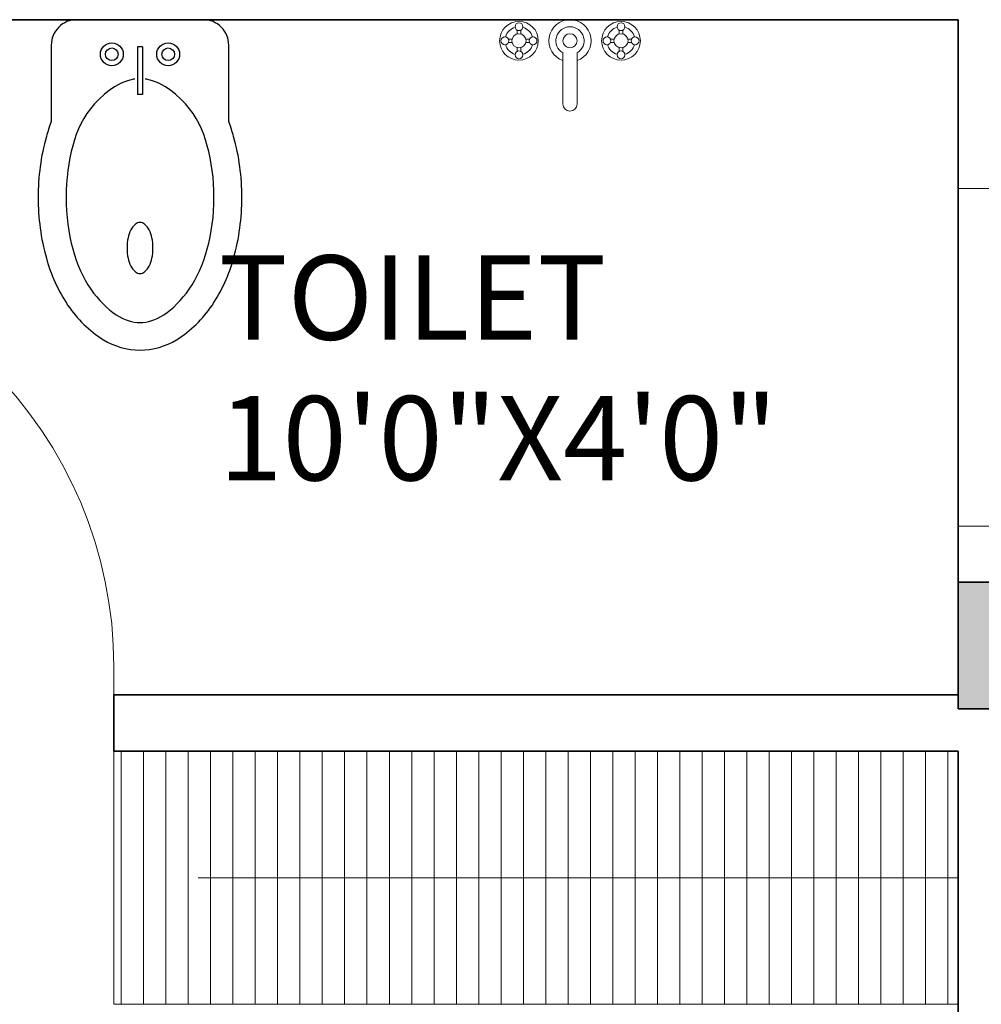
# Model space of a CAD drawing. Units: inches. Extents: x 3321 to 5237, y 11 to 1752.
# Tile 8 of 43: x 3725 to 3793, y 1298 to 1368. Entities that reach past the tile are written whole.
import ezdxf

# ---------------------------------------------------------------- set-up
doc = ezdxf.new("R2010")
doc.units = ezdxf.units.IN
for name, color, linetype, lineweight in [('A-AREA-IDEN', 7, 'Continuous', 18), ('A-COLS', 1, 'Continuous', 35), ('A-DOOR', 4, 'Continuous', 18), ('A-FLOR-CASE', 8, 'Continuous', 18), ('A-FLOR-CASE-PATT', 8, 'Continuous', 13), ('A-GLAZ', 5, 'Continuous', 18), ('A-WALL', 7, 'Continuous', 35), ('Сантехника', 7, 'Continuous', 18)]:
    doc.layers.add(name, color=color, linetype=linetype, lineweight=lineweight)
doc.layers.add('SANTEH', color=7, linetype='Continuous')
doc.styles.get("Standard").update_dxf_attribs({"font": 'arial.ttf'})

# ---------------------------------------------------------------- blocks, each defined once
blk = doc.blocks.new('*U6')
for p, q in [((-30, 0), (-30, 6)), ((0, 0), (0, 6))]:
    blk.add_line(p, q)
blk.add_lwpolyline([(0, 0), (0, -30), (-1.75, -30), (-1.75, 0)], close=True)
blk.add_arc((0, 0), 30, 180, 270)
blk = doc.blocks.new('K10-45')
at = {"layer": 'SANTEH'}
for p, q in [((-18.9, 83.4), (-18.9, 177.1)), ((-18.9, 177.1), (-8.9, 177.1)), ((-8.9, 83.4), (-8.9, 177.1)), ((-18.9, 83.4), (-8.9, 83.4))]:
    blk.add_line(p, q, dxfattribs=at)
for points in [[(160.3, 230.4, 0.023928), (169.9, 259.6, 0.067459), (186.1, 379, 0.067459), (169.9, 498.4, 0.079812), (127.5, 591.1, 0.107118), (58, 658.5, 0.139889), (-13.9, 679, 0.139889), (-85.8, 658.5, 0.107118), (-155.3, 591.1, 0.079812), (-197.7, 498.4, 0.067459), (-213.9, 379, 0.067459), (-197.7, 259.6, 0.023928), (-188.1, 230.4), (-188.1, 80.2, 0.414214), (-138.1, 30.2), (110.3, 30.2, 0.414214), (160.3, 80.2)], [(-39.4, 478.5, 0.052061), (-37.3, 458.3, 0.065919), (-32, 443.1, 0.104629), (-22.6, 431.5, 0.172287), (-13.9, 428.4, 0.172287), (-5.2, 431.5, 0.104629), (4.1, 443.1, 0.065919), (9.5, 458.3, 0.052061), (11.6, 478.5, 0.052061), (9.5, 498.7, 0.065919), (4.1, 513.9, 0.104629), (-5.2, 525.5, 0.172287), (-13.9, 528.6, 0.172287), (-22.6, 525.5, 0.104629), (-32, 513.9, 0.065919), (-37.3, 498.7, 0.052061)]]:
    blk.add_lwpolyline(points, format="xyb", close=True, dxfattribs=at)
blk.add_lwpolyline([(-3.9, 147), (-1.4, 147.2), (10.9, 150.3), (23, 155.1), (34.7, 161.4), (45.9, 168.8), (56.5, 177.2), (66.3, 186.2), (75.2, 195.5), (83.2, 205), (90.3, 214.7), (96.5, 224.5), (102, 234.5), (106.9, 244.7), (111.1, 255.3), (114.8, 266.2), (118.1, 277.6), (121.1, 289.3), (123.7, 301.4), (126, 313.8), (127.9, 326.5), (129.3, 339.5), (130.4, 352.6), (131.1, 365.8), (131.3, 379), (131.1, 392.2), (130.4, 405.4), (129.3, 418.5), (127.9, 431.4), (126, 444.2), (123.7, 456.6), (121.1, 468.7), (118.1, 480.4), (114.8, 491.7), (111.2, 502.6), (107.3, 513.1), (103, 523.1), (98.4, 532.7), (93.5, 541.9), (88.3, 550.7), (82.8, 559.1), (77.1, 567.1), (71, 574.6), (64.9, 581.7), (58.5, 588.3), (52.1, 594.4), (45.7, 600), (39.3, 605), (33, 609.4), (26.9, 613.2), (20.8, 616.4), (14.9, 619), (9, 621.1), (3.2, 622.7), (-2.5, 623.8), (-8.2, 624.5), (-13.9, 624.7), (-19.6, 624.5), (-25.3, 623.8), (-31, 622.7), (-36.8, 621.1), (-42.7, 619), (-48.6, 616.4), (-54.7, 613.2), (-60.9, 609.4), (-67.2, 605), (-73.5, 600), (-80, 594.4), (-86.4, 588.3), (-92.7, 581.7), (-98.9, 574.6), (-104.9, 567.1), (-110.6, 559.1), (-116.1, 550.7), (-121.3, 541.9), (-126.2, 532.7), (-130.8, 523.1), (-135.1, 513.1), (-139, 502.6), (-142.7, 491.7), (-146, 480.4), (-148.9, 468.7), (-151.5, 456.6), (-153.8, 444.2), (-155.7, 431.4), (-157.2, 418.5), (-158.2, 405.4), (-158.9, 392.2), (-159.1, 379), (-158.9, 365.8), (-158.2, 352.6), (-157.2, 339.5), (-155.7, 326.5), (-153.8, 313.8), (-151.5, 301.4), (-148.9, 289.3), (-146, 277.6), (-142.6, 266.2), (-138.9, 255.3), (-134.7, 244.7), (-129.8, 234.5), (-124.4, 224.5), (-118.1, 214.7), (-111, 205), (-103.1, 195.5), (-94.1, 186.2), (-84.3, 177.2), (-73.7, 168.8), (-62.5, 161.4), (-50.8, 155.1), (-38.7, 150.3), (-26.4, 147.2), (-23.9, 147)], dxfattribs=at)
for centre, radius in [((-69.2, 98.1), 22.4), ((41.4, 98.1), 22.4), ((-69.2, 98.1), 12.4), ((41.4, 98.1), 12.4)]:
    blk.add_circle(centre, radius, dxfattribs=at)
blk = doc.blocks.new('Faucet - Bathroom top')
for p, q in [((-3.75, 0.4788), (-3.75, 0.75)), ((-3.5, 0.482), (-3.5, 0.75)), ((3.5, 0.4788), (3.5, 0.75)), ((3.75, 0.482), (3.75, 0.75)), ((-4.107, 0.125), (-4.375, 0.125)), ((-3.1461, 0.125), (-2.875, 0.125)), ((3.143, 0.125), (2.875, 0.125)), ((4.1039, 0.125), (4.375, 0.125)), ((-4.1039, -0.125), (-4.375, -0.125)), ((-3.75, -0.4821), (-3.75, -0.75)), ((-3.5, -0.4789), (-3.5, -0.75)), ((-3.143, -0.125), (-2.875, -0.125)), ((3.1461, -0.125), (2.875, -0.125)), ((3.5, -0.4821), (3.5, -0.75)), ((3.75, -0.4789), (3.75, -0.75)), ((4.107, -0.125), (4.375, -0.125)), ((-0.5, -0.8639), (-0.5, -4.5)), ((0.5, -4.5), (0.5, -0.8631))]:
    blk.add_line(p, q)
for centre, radius in [((-3.625, 0), 1.375), ((-3.625, 1), 0.2795), ((3.625, 0), 1.375), ((3.625, 1), 0.2795), ((-4.625, 0), 0.2795), ((-3.625, 0), 0.5), ((-2.625, 0), 0.2795), ((0, 0), 0.5), ((2.625, 0), 0.2795), ((3.625, 0), 0.5), ((4.625, 0), 0.2795), ((-3.625, -1), 0.2795), ((3.625, -1), 0.2795)]:
    blk.add_circle(centre, radius)
for centre, radius, start, end in [((0, 0), 1.5, 289.6514, 250.3603), ((-3.625, 0), 1, 105.2407, 164.2093), ((-3.625, 0), 1, 16.44125, 74.07887), ((0, 0), 1, 300.3431, 239.7554), ((3.625, 0), 1, 106.12, 164.0884), ((3.625, 0), 1, 16.23422, 73.90469), ((-3.625, 0), 1, 196.2342, 253.9047), ((-3.625, 0), 1, 286.12, 344.0884), ((3.625, 0), 1, 196.4413, 254.0789), ((3.625, 0), 1, 285.2407, 344.2093), ((0, -4.5), 0.5, 180, 0)]:
    blk.add_arc(centre, radius, start, end)
blk = doc.blocks.new('COL-9X9-FURN-PLAN')
h = blk.add_hatch(color=256)
h.dxf.hatch_style = 1
h.paths.add_polyline_path([(9, 9), (0, 9), (0, 0), (9, 0)])
blk.add_lwpolyline([(0, 0), (9, 0), (9, 9), (0, 9)], close=True)
blk = doc.blocks.new('WIN-24IN-9IN-WALL')
for p, q in [((9, 24), (0, 24)), ((4, 24), (4, 0)), ((5, 24), (5, 0)), ((9, 0), (0, 0))]:
    blk.add_line(p, q)

msp = doc.modelspace()

# ---------------------------------------------------------------- hatches: boundary and pattern name
at = {"layer": 'A-FLOR-CASE-PATT'}
h = msp.add_hatch(dxfattribs=at)
h.set_pattern_fill('ANSI31', color=256, scale=0.5, angle=45)
h.paths.add_polyline_path([(3791.689, 1316.339), (3731.689, 1316.339), (3731.689, 1298.339), (3791.689, 1298.339)])

# ---------------------------------------------------------------- linework, layer by layer
at = {"layer": 'A-FLOR-CASE'}
for p, q in [((3731.689, 1316.339), (3731.689, 1298.339)), ((3737.689, 1307.339), (3791.689, 1307.339)), ((3731.689, 1298.339), (3791.689, 1298.339))]:
    msp.add_line(p, q, dxfattribs=at)
at = {"layer": 'A-WALL'}
for p, q in [((3671.689, 1368.339), (3791.689, 1368.339)), ((3791.689, 1368.339), (3791.689, 1320.339)), ((3731.689, 1320.339), (3731.689, 1316.339)), ((3731.689, 1320.339), (3791.689, 1320.339)), ((3731.689, 1316.339), (3791.689, 1316.339)), ((3791.689, 1316.339), (3791.689, 1181.339))]:
    msp.add_line(p, q, dxfattribs=at)

# ---------------------------------------------------------------- block references
at = {"layer": 'A-COLS'}
msp.add_blockref('COL-9X9-FURN-PLAN', (3791.689, 1319.339), dxfattribs=at)
at = {"layer": 'A-DOOR', "rotation": 180}
msp.add_blockref('*U6', (3701.689, 1322.339), dxfattribs=at)
at = {"layer": 'A-GLAZ'}
msp.add_blockref('WIN-24IN-9IN-WALL', (3791.689, 1332.339), dxfattribs=at)
at = {"layer": 'Сантехника', "xscale": 0.0362080263207385, "yscale": 0.0362080263207385, "zscale": 0.0362080263207385, "rotation": 180}
msp.add_blockref('K10-45', (3733.044, 1369.432), dxfattribs=at)
at = {"layer": 'Сантехника', "xscale": -1}
msp.add_blockref('Faucet - Bathroom top', (3764.1, 1366.839), dxfattribs=at)

# ---------------------------------------------------------------- texts
at = {"layer": 'A-AREA-IDEN', "insert": (3739.14, 1351.587), "char_height": 6, "attachment_point": 1}
msp.add_mtext_dynamic_manual_height_columns('TOILET\\P10\'0"X4\'0"', width=97.3114, gutter_width=25, heights=[0], dxfattribs=at)

doc.saveas('drawing.dxf')
